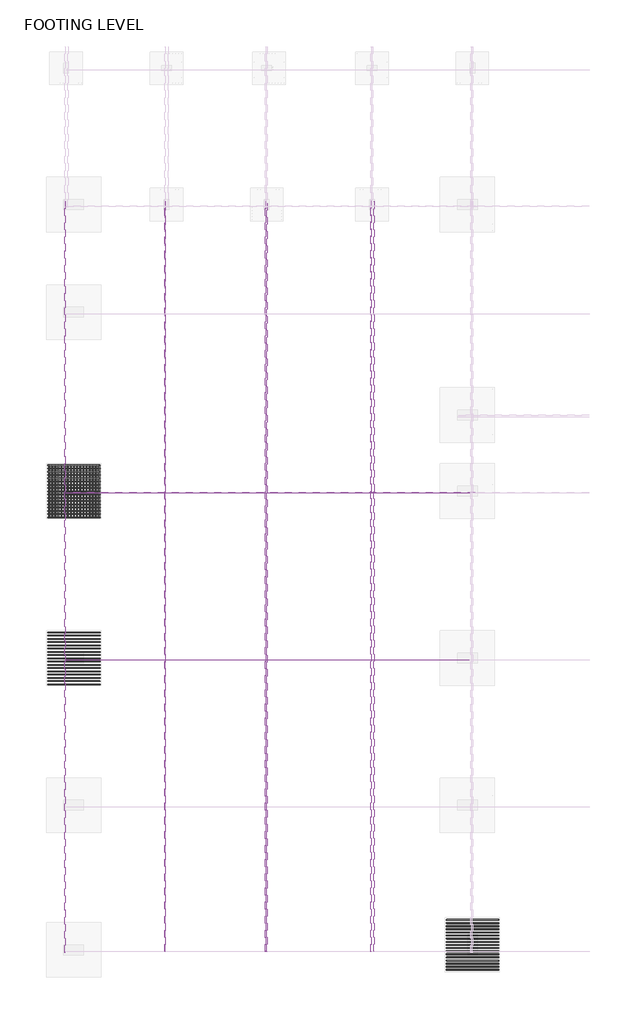
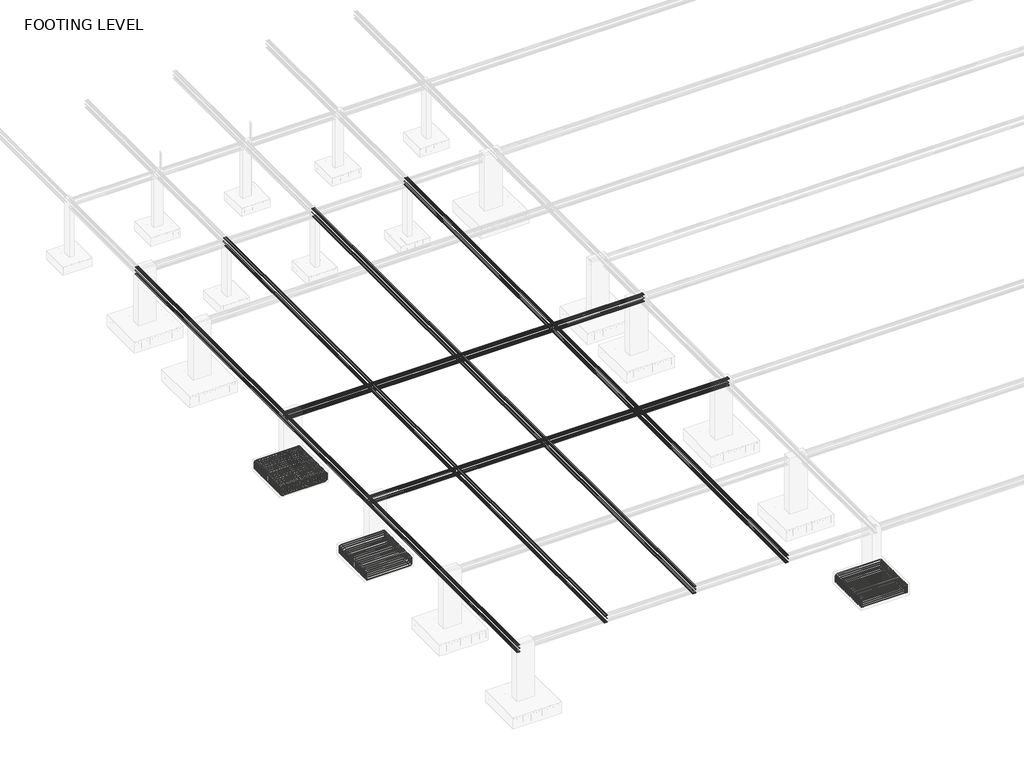
# One storey, part 4 of 19: 26 reinforcing bars.
"""IFC4 building model written with IfcOpenShell, lengths in millimetres."""

from ifc_helpers import new_model, si_unit, point, frame, origin, place, context, project, spatial, polyline, circle_curve, trimmed, segment, composite_curve, source, transform, mapped, element, save
from ifc_brep_helpers import swept_disk

model = new_model("IFC4")

# Units and contexts
model_context = context("Model", 3, world=origin())
ifc_project = project(units=[si_unit("LENGTHUNIT", "METRE", prefix="MILLI")], contexts=[model_context])

# Site, building, storey
site = spatial("IfcSite", under=ifc_project)
building = spatial("IfcBuilding", under=site)
storey = spatial("IfcBuildingStorey", under=building, Name="FOOTING LEVEL", Elevation=-3048.0)

# Reinforcing bars
placement = place(None, origin())
reinforcing_bar_shape = source(origin(), model_context, "Body", "SolidModel", [
    swept_disk(composite_curve([segment(polyline([(2562.6587563, -28952.7516566, -3148.0), (2562.6587563, -28952.7516566, -3470.1)]), True, "CONTINUOUS"), segment(trimmed(circle_curve(frame((2472.4587563, -28952.7516566, -3470.1), z_axis=(0.0, 1.0, 0.0), x_axis=(90.19999999999982, 0.0, 0.0)), 90.2), [point((2562.6587563, -28952.7516566, -3470.1))], [point((2472.4587563, -28952.7516566, -3560.3))], True, "CARTESIAN"), True, "CONTINUOUS"), segment(polyline([(2472.4587563, -28952.7516566, -3560.3), (278.2587563, -28952.7516566, -3560.3)]), True, "CONTINUOUS"), segment(trimmed(circle_curve(frame((278.2587563, -28952.7516566, -3470.1), z_axis=(0.0, 1.0, 0.0), x_axis=(0.0, 0.0, -90.20000000000027)), 90.2), [point((278.2587563, -28952.7516566, -3560.3))], [point((188.0587563, -28952.7516566, -3470.1))], True, "CARTESIAN"), True, "CONTINUOUS"), segment(polyline([(188.0587563, -28952.7516566, -3470.1), (188.0587563, -28952.7516566, -3148.0)]), True, "CONTINUOUS")], self_intersect=False), 12.7),
])
element("IfcReinforcingBar", 1, at=placement, inside=storey, context=model_context, shape_type="MappedRepresentation", body=[
    mapped(reinforcing_bar_shape, transform((0.0, 0.0, 0.0), x_axis=(1.0, 0.0, 0.0), y_axis=(0.0, 1.0, 0.0), z_axis=(0.0, 0.0, 1.0))),
    mapped(reinforcing_bar_shape, transform((0.0, 140.8090411, 0.0), x_axis=(1.0, 0.0, 0.0), y_axis=(0.0, 1.0, 0.0), z_axis=(0.0, 0.0, 1.0))),
    mapped(reinforcing_bar_shape, transform((0.0, 281.6180821, 0.0), x_axis=(1.0, 0.0, 0.0), y_axis=(0.0, 1.0, 0.0), z_axis=(0.0, 0.0, 1.0))),
    mapped(reinforcing_bar_shape, transform((0.0, 422.4271232, 0.0), x_axis=(1.0, 0.0, 0.0), y_axis=(0.0, 1.0, 0.0), z_axis=(0.0, 0.0, 1.0))),
    mapped(reinforcing_bar_shape, transform((0.0, 563.2361643, 0.0), x_axis=(1.0, 0.0, 0.0), y_axis=(0.0, 1.0, 0.0), z_axis=(0.0, 0.0, 1.0))),
    mapped(reinforcing_bar_shape, transform((0.0, 704.0452054, 0.0), x_axis=(1.0, 0.0, 0.0), y_axis=(0.0, 1.0, 0.0), z_axis=(0.0, 0.0, 1.0))),
    mapped(reinforcing_bar_shape, transform((0.0, 844.8542464, 0.0), x_axis=(1.0, 0.0, 0.0), y_axis=(0.0, 1.0, 0.0), z_axis=(0.0, 0.0, 1.0))),
    mapped(reinforcing_bar_shape, transform((0.0, 985.6632875, 0.0), x_axis=(1.0, 0.0, 0.0), y_axis=(0.0, 1.0, 0.0), z_axis=(0.0, 0.0, 1.0))),
    mapped(reinforcing_bar_shape, transform((0.0, 1126.4723286, 0.0), x_axis=(1.0, 0.0, 0.0), y_axis=(0.0, 1.0, 0.0), z_axis=(0.0, 0.0, 1.0))),
    mapped(reinforcing_bar_shape, transform((0.0, 1267.2813697, 0.0), x_axis=(1.0, 0.0, 0.0), y_axis=(0.0, 1.0, 0.0), z_axis=(0.0, 0.0, 1.0))),
    mapped(reinforcing_bar_shape, transform((0.0, 1408.0904107, 0.0), x_axis=(1.0, 0.0, 0.0), y_axis=(0.0, 1.0, 0.0), z_axis=(0.0, 0.0, 1.0))),
    mapped(reinforcing_bar_shape, transform((0.0, 1548.8994518, 0.0), x_axis=(1.0, 0.0, 0.0), y_axis=(0.0, 1.0, 0.0), z_axis=(0.0, 0.0, 1.0))),
    mapped(reinforcing_bar_shape, transform((0.0, 1689.7084929, 0.0), x_axis=(1.0, 0.0, 0.0), y_axis=(0.0, 1.0, 0.0), z_axis=(0.0, 0.0, 1.0))),
    mapped(reinforcing_bar_shape, transform((0.0, 1830.517534, 0.0), x_axis=(1.0, 0.0, 0.0), y_axis=(0.0, 1.0, 0.0), z_axis=(0.0, 0.0, 1.0))),
    mapped(reinforcing_bar_shape, transform((0.0, 1971.326575, 0.0), x_axis=(1.0, 0.0, 0.0), y_axis=(0.0, 1.0, 0.0), z_axis=(0.0, 0.0, 1.0))),
    mapped(reinforcing_bar_shape, transform((0.0, 2112.1356161, 0.0), x_axis=(1.0, 0.0, 0.0), y_axis=(0.0, 1.0, 0.0), z_axis=(0.0, 0.0, 1.0))),
    mapped(reinforcing_bar_shape, transform((0.0, 2252.9446572, 0.0), x_axis=(1.0, 0.0, 0.0), y_axis=(0.0, 1.0, 0.0), z_axis=(0.0, 0.0, 1.0))),
])
reinforcing_bar_2_shape = source(origin(), model_context, "Body", "SolidModel", [
    swept_disk(composite_curve([segment(polyline([(2562.6587563, -26677.3596072, -3548.0), (2562.6587563, -26677.3596072, -3225.9)]), True, "CONTINUOUS"), segment(trimmed(circle_curve(frame((2472.4587563, -26677.3596072, -3225.9), z_axis=(0.0, -1.0, 0.0), x_axis=(90.19999999999982, 0.0, 0.0)), 90.2), [point((2562.6587563, -26677.3596072, -3225.9))], [point((2472.4587563, -26677.3596072, -3135.7))], True, "CARTESIAN"), True, "CONTINUOUS"), segment(polyline([(2472.4587563, -26677.3596072, -3135.7), (278.2587563, -26677.3596072, -3135.7)]), True, "CONTINUOUS"), segment(trimmed(circle_curve(frame((278.2587563, -26677.3596072, -3225.9), z_axis=(0.0, -1.0, 0.0), x_axis=(0.0, 0.0, 90.20000000000027)), 90.2), [point((278.2587563, -26677.3596072, -3135.7))], [point((188.0587563, -26677.3596072, -3225.9))], True, "CARTESIAN"), True, "CONTINUOUS"), segment(polyline([(188.0587563, -26677.3596072, -3225.9), (188.0587563, -26677.3596072, -3548.0)]), True, "CONTINUOUS")], self_intersect=False), 12.7),
])
element("IfcReinforcingBar", 2, at=placement, inside=storey, context=model_context, shape_type="MappedRepresentation", body=[
    mapped(reinforcing_bar_2_shape, transform((0.0, 0.0, 0.0), x_axis=(1.0, 0.0, 0.0), y_axis=(0.0, 1.0, 0.0), z_axis=(0.0, 0.0, 1.0))),
    mapped(reinforcing_bar_2_shape, transform((0.0, -143.8496077, 0.0), x_axis=(1.0, 0.0, 0.0), y_axis=(0.0, 1.0, 0.0), z_axis=(0.0, 0.0, 1.0))),
    mapped(reinforcing_bar_2_shape, transform((0.0, -287.6992155, 0.0), x_axis=(1.0, 0.0, 0.0), y_axis=(0.0, 1.0, 0.0), z_axis=(0.0, 0.0, 1.0))),
    mapped(reinforcing_bar_2_shape, transform((0.0, -431.5488232, 0.0), x_axis=(1.0, 0.0, 0.0), y_axis=(0.0, 1.0, 0.0), z_axis=(0.0, 0.0, 1.0))),
    mapped(reinforcing_bar_2_shape, transform((0.0, -575.398431, 0.0), x_axis=(1.0, 0.0, 0.0), y_axis=(0.0, 1.0, 0.0), z_axis=(0.0, 0.0, 1.0))),
    mapped(reinforcing_bar_2_shape, transform((0.0, -719.2480387, 0.0), x_axis=(1.0, 0.0, 0.0), y_axis=(0.0, 1.0, 0.0), z_axis=(0.0, 0.0, 1.0))),
    mapped(reinforcing_bar_2_shape, transform((0.0, -863.0976465, 0.0), x_axis=(1.0, 0.0, 0.0), y_axis=(0.0, 1.0, 0.0), z_axis=(0.0, 0.0, 1.0))),
    mapped(reinforcing_bar_2_shape, transform((0.0, -1006.9472542, 0.0), x_axis=(1.0, 0.0, 0.0), y_axis=(0.0, 1.0, 0.0), z_axis=(0.0, 0.0, 1.0))),
    mapped(reinforcing_bar_2_shape, transform((0.0, -1150.796862, 0.0), x_axis=(1.0, 0.0, 0.0), y_axis=(0.0, 1.0, 0.0), z_axis=(0.0, 0.0, 1.0))),
    mapped(reinforcing_bar_2_shape, transform((0.0, -1294.6464697, 0.0), x_axis=(1.0, 0.0, 0.0), y_axis=(0.0, 1.0, 0.0), z_axis=(0.0, 0.0, 1.0))),
    mapped(reinforcing_bar_2_shape, transform((0.0, -1438.4960775, 0.0), x_axis=(1.0, 0.0, 0.0), y_axis=(0.0, 1.0, 0.0), z_axis=(0.0, 0.0, 1.0))),
    mapped(reinforcing_bar_2_shape, transform((0.0, -1582.3456852, 0.0), x_axis=(1.0, 0.0, 0.0), y_axis=(0.0, 1.0, 0.0), z_axis=(0.0, 0.0, 1.0))),
    mapped(reinforcing_bar_2_shape, transform((0.0, -1726.195293, 0.0), x_axis=(1.0, 0.0, 0.0), y_axis=(0.0, 1.0, 0.0), z_axis=(0.0, 0.0, 1.0))),
    mapped(reinforcing_bar_2_shape, transform((0.0, -1870.0449007, 0.0), x_axis=(1.0, 0.0, 0.0), y_axis=(0.0, 1.0, 0.0), z_axis=(0.0, 0.0, 1.0))),
    mapped(reinforcing_bar_2_shape, transform((0.0, -2013.8945085, 0.0), x_axis=(1.0, 0.0, 0.0), y_axis=(0.0, 1.0, 0.0), z_axis=(0.0, 0.0, 1.0))),
    mapped(reinforcing_bar_2_shape, transform((0.0, -2157.7441162, 0.0), x_axis=(1.0, 0.0, 0.0), y_axis=(0.0, 1.0, 0.0), z_axis=(0.0, 0.0, 1.0))),
    mapped(reinforcing_bar_2_shape, transform((0.0, -2301.5937239, 0.0), x_axis=(1.0, 0.0, 0.0), y_axis=(0.0, 1.0, 0.0), z_axis=(0.0, 0.0, 1.0))),
])
reinforcing_bar_3_shape = source(origin(), model_context, "Body", "SolidModel", [
    swept_disk(composite_curve([segment(polyline([(-17985.6412437, -13575.4205555, -3173.0), (-17985.6412437, -13575.4205555, -3495.1)]), True, "CONTINUOUS"), segment(trimmed(circle_curve(frame((-17895.4412437, -13575.4205555, -3495.1), z_axis=(0.0, -1.0, 0.0), x_axis=(-90.20000000000073, 0.0, 0.0)), 90.2), [point((-17985.6412437, -13575.4205555, -3495.1))], [point((-17895.4412437, -13575.4205555, -3585.3))], True, "CARTESIAN"), True, "CONTINUOUS"), segment(polyline([(-17895.4412437, -13575.4205555, -3585.3), (-15701.2412437, -13575.4205555, -3585.3)]), True, "CONTINUOUS"), segment(trimmed(circle_curve(frame((-15701.2412437, -13575.4205555, -3495.1), z_axis=(0.0, -1.0, 0.0), x_axis=(0.0, 0.0, -90.20000000000027)), 90.2), [point((-15701.2412437, -13575.4205555, -3585.3))], [point((-15611.0412437, -13575.4205555, -3495.1))], True, "CARTESIAN"), True, "CONTINUOUS"), segment(polyline([(-15611.0412437, -13575.4205555, -3495.1), (-15611.0412437, -13575.4205555, -3173.0)]), True, "CONTINUOUS")], self_intersect=False), 12.7),
])
element("IfcReinforcingBar", 3, at=placement, inside=storey, context=model_context, shape_type="MappedRepresentation", body=[
    mapped(reinforcing_bar_3_shape, transform((0.0, 0.0, 0.0), x_axis=(1.0, 0.0, 0.0), y_axis=(0.0, 1.0, 0.0), z_axis=(0.0, 0.0, 1.0))),
    mapped(reinforcing_bar_3_shape, transform((0.0, -148.4125, 0.0), x_axis=(1.0, 0.0, 0.0), y_axis=(0.0, 1.0, 0.0), z_axis=(0.0, 0.0, 1.0))),
    mapped(reinforcing_bar_3_shape, transform((0.0, -296.825, 0.0), x_axis=(1.0, 0.0, 0.0), y_axis=(0.0, 1.0, 0.0), z_axis=(0.0, 0.0, 1.0))),
    mapped(reinforcing_bar_3_shape, transform((0.0, -445.2375, 0.0), x_axis=(1.0, 0.0, 0.0), y_axis=(0.0, 1.0, 0.0), z_axis=(0.0, 0.0, 1.0))),
    mapped(reinforcing_bar_3_shape, transform((0.0, -593.65, 0.0), x_axis=(1.0, 0.0, 0.0), y_axis=(0.0, 1.0, 0.0), z_axis=(0.0, 0.0, 1.0))),
    mapped(reinforcing_bar_3_shape, transform((0.0, -742.0625, 0.0), x_axis=(1.0, 0.0, 0.0), y_axis=(0.0, 1.0, 0.0), z_axis=(0.0, 0.0, 1.0))),
    mapped(reinforcing_bar_3_shape, transform((0.0, -890.475, 0.0), x_axis=(1.0, 0.0, 0.0), y_axis=(0.0, 1.0, 0.0), z_axis=(0.0, 0.0, 1.0))),
    mapped(reinforcing_bar_3_shape, transform((0.0, -1038.8875, 0.0), x_axis=(1.0, 0.0, 0.0), y_axis=(0.0, 1.0, 0.0), z_axis=(0.0, 0.0, 1.0))),
    mapped(reinforcing_bar_3_shape, transform((0.0, -1187.3, 0.0), x_axis=(1.0, 0.0, 0.0), y_axis=(0.0, 1.0, 0.0), z_axis=(0.0, 0.0, 1.0))),
    mapped(reinforcing_bar_3_shape, transform((0.0, -1335.7125, 0.0), x_axis=(1.0, 0.0, 0.0), y_axis=(0.0, 1.0, 0.0), z_axis=(0.0, 0.0, 1.0))),
    mapped(reinforcing_bar_3_shape, transform((0.0, -1484.125, 0.0), x_axis=(1.0, 0.0, 0.0), y_axis=(0.0, 1.0, 0.0), z_axis=(0.0, 0.0, 1.0))),
    mapped(reinforcing_bar_3_shape, transform((0.0, -1632.5375, 0.0), x_axis=(1.0, 0.0, 0.0), y_axis=(0.0, 1.0, 0.0), z_axis=(0.0, 0.0, 1.0))),
    mapped(reinforcing_bar_3_shape, transform((0.0, -1780.95, 0.0), x_axis=(1.0, 0.0, 0.0), y_axis=(0.0, 1.0, 0.0), z_axis=(0.0, 0.0, 1.0))),
    mapped(reinforcing_bar_3_shape, transform((0.0, -1929.3625, 0.0), x_axis=(1.0, 0.0, 0.0), y_axis=(0.0, 1.0, 0.0), z_axis=(0.0, 0.0, 1.0))),
    mapped(reinforcing_bar_3_shape, transform((0.0, -2077.775, 0.0), x_axis=(1.0, 0.0, 0.0), y_axis=(0.0, 1.0, 0.0), z_axis=(0.0, 0.0, 1.0))),
    mapped(reinforcing_bar_3_shape, transform((0.0, -2226.1875, 0.0), x_axis=(1.0, 0.0, 0.0), y_axis=(0.0, 1.0, 0.0), z_axis=(0.0, 0.0, 1.0))),
    mapped(reinforcing_bar_3_shape, transform((0.0, -2374.6, 0.0), x_axis=(1.0, 0.0, 0.0), y_axis=(0.0, 1.0, 0.0), z_axis=(0.0, 0.0, 1.0))),
])
reinforcing_bar_4_shape = source(origin(), model_context, "Body", "SolidModel", [
    swept_disk(composite_curve([segment(polyline([(-15611.0412437, -13575.4205555, -3523.0), (-15611.0412437, -13575.4205555, -3200.9)]), True, "CONTINUOUS"), segment(trimmed(circle_curve(frame((-15701.2412437, -13575.4205555, -3200.9), z_axis=(0.0, -1.0, 0.0), x_axis=(90.20000000000073, 0.0, 0.0)), 90.2), [point((-15611.0412437, -13575.4205555, -3200.9))], [point((-15701.2412437, -13575.4205555, -3110.7))], True, "CARTESIAN"), True, "CONTINUOUS"), segment(polyline([(-15701.2412437, -13575.4205555, -3110.7), (-17895.4412437, -13575.4205555, -3110.7)]), True, "CONTINUOUS"), segment(trimmed(circle_curve(frame((-17895.4412437, -13575.4205555, -3200.9), z_axis=(0.0, -1.0, 0.0), x_axis=(0.0, 0.0, 90.20000000000027)), 90.2), [point((-17895.4412437, -13575.4205555, -3110.7))], [point((-17985.6412437, -13575.4205555, -3200.9))], True, "CARTESIAN"), True, "CONTINUOUS"), segment(polyline([(-17985.6412437, -13575.4205555, -3200.9), (-17985.6412437, -13575.4205555, -3523.0)]), True, "CONTINUOUS")], self_intersect=False), 12.7),
])
element("IfcReinforcingBar", 4, at=placement, inside=storey, context=model_context, shape_type="MappedRepresentation", body=[
    mapped(reinforcing_bar_4_shape, transform((0.0, 0.0, 0.0), x_axis=(1.0, 0.0, 0.0), y_axis=(0.0, 1.0, 0.0), z_axis=(0.0, 0.0, 1.0))),
    mapped(reinforcing_bar_4_shape, transform((0.0, -148.4125, 0.0), x_axis=(1.0, 0.0, 0.0), y_axis=(0.0, 1.0, 0.0), z_axis=(0.0, 0.0, 1.0))),
    mapped(reinforcing_bar_4_shape, transform((0.0, -296.825, 0.0), x_axis=(1.0, 0.0, 0.0), y_axis=(0.0, 1.0, 0.0), z_axis=(0.0, 0.0, 1.0))),
    mapped(reinforcing_bar_4_shape, transform((0.0, -445.2375, 0.0), x_axis=(1.0, 0.0, 0.0), y_axis=(0.0, 1.0, 0.0), z_axis=(0.0, 0.0, 1.0))),
    mapped(reinforcing_bar_4_shape, transform((0.0, -593.65, 0.0), x_axis=(1.0, 0.0, 0.0), y_axis=(0.0, 1.0, 0.0), z_axis=(0.0, 0.0, 1.0))),
    mapped(reinforcing_bar_4_shape, transform((0.0, -742.0625, 0.0), x_axis=(1.0, 0.0, 0.0), y_axis=(0.0, 1.0, 0.0), z_axis=(0.0, 0.0, 1.0))),
    mapped(reinforcing_bar_4_shape, transform((0.0, -890.475, 0.0), x_axis=(1.0, 0.0, 0.0), y_axis=(0.0, 1.0, 0.0), z_axis=(0.0, 0.0, 1.0))),
    mapped(reinforcing_bar_4_shape, transform((0.0, -1038.8875, 0.0), x_axis=(1.0, 0.0, 0.0), y_axis=(0.0, 1.0, 0.0), z_axis=(0.0, 0.0, 1.0))),
    mapped(reinforcing_bar_4_shape, transform((0.0, -1187.3, 0.0), x_axis=(1.0, 0.0, 0.0), y_axis=(0.0, 1.0, 0.0), z_axis=(0.0, 0.0, 1.0))),
    mapped(reinforcing_bar_4_shape, transform((0.0, -1335.7125, 0.0), x_axis=(1.0, 0.0, 0.0), y_axis=(0.0, 1.0, 0.0), z_axis=(0.0, 0.0, 1.0))),
    mapped(reinforcing_bar_4_shape, transform((0.0, -1484.125, 0.0), x_axis=(1.0, 0.0, 0.0), y_axis=(0.0, 1.0, 0.0), z_axis=(0.0, 0.0, 1.0))),
    mapped(reinforcing_bar_4_shape, transform((0.0, -1632.5375, 0.0), x_axis=(1.0, 0.0, 0.0), y_axis=(0.0, 1.0, 0.0), z_axis=(0.0, 0.0, 1.0))),
    mapped(reinforcing_bar_4_shape, transform((0.0, -1780.95, 0.0), x_axis=(1.0, 0.0, 0.0), y_axis=(0.0, 1.0, 0.0), z_axis=(0.0, 0.0, 1.0))),
    mapped(reinforcing_bar_4_shape, transform((0.0, -1929.3625, 0.0), x_axis=(1.0, 0.0, 0.0), y_axis=(0.0, 1.0, 0.0), z_axis=(0.0, 0.0, 1.0))),
    mapped(reinforcing_bar_4_shape, transform((0.0, -2077.775, 0.0), x_axis=(1.0, 0.0, 0.0), y_axis=(0.0, 1.0, 0.0), z_axis=(0.0, 0.0, 1.0))),
    mapped(reinforcing_bar_4_shape, transform((0.0, -2226.1875, 0.0), x_axis=(1.0, 0.0, 0.0), y_axis=(0.0, 1.0, 0.0), z_axis=(0.0, 0.0, 1.0))),
    mapped(reinforcing_bar_4_shape, transform((0.0, -2374.6, 0.0), x_axis=(1.0, 0.0, 0.0), y_axis=(0.0, 1.0, 0.0), z_axis=(0.0, 0.0, 1.0))),
])
reinforcing_bar_5_shape = source(origin(), model_context, "Body", "SolidModel", [
    swept_disk(composite_curve([segment(polyline([(-17920.0723448, -8330.0205555, -3148.0), (-17920.0723448, -8330.0205555, -3470.1)]), True, "CONTINUOUS"), segment(trimmed(circle_curve(frame((-17920.0723448, -8239.8205555, -3470.1), z_axis=(1.0, 0.0, 0.0), x_axis=(0.0, -90.19999999999891, 0.0)), 90.2), [point((-17920.0723448, -8330.0205555, -3470.1))], [point((-17920.0723448, -8239.8205555, -3560.3))], True, "CARTESIAN"), True, "CONTINUOUS"), segment(polyline([(-17920.0723448, -8239.8205555, -3560.3), (-17920.0723448, -6045.6205555, -3560.3)]), True, "CONTINUOUS"), segment(trimmed(circle_curve(frame((-17920.0723448, -6045.6205555, -3470.1), z_axis=(1.0, 0.0, 0.0), x_axis=(0.0, 0.0, -90.20000000000027)), 90.2), [point((-17920.0723448, -6045.6205555, -3560.3))], [point((-17920.0723448, -5955.4205555, -3470.1))], True, "CARTESIAN"), True, "CONTINUOUS"), segment(polyline([(-17920.0723448, -5955.4205555, -3470.1), (-17920.0723448, -5955.4205555, -3148.0)]), True, "CONTINUOUS")], self_intersect=False), 12.7),
])
element("IfcReinforcingBar", 5, at=placement, inside=storey, context=model_context, shape_type="MappedRepresentation", body=[
    mapped(reinforcing_bar_5_shape, transform((0.0, 0.0, 0.0), x_axis=(1.0, 0.0, 0.0), y_axis=(0.0, 1.0, 0.0), z_axis=(0.0, 0.0, 1.0))),
    mapped(reinforcing_bar_5_shape, transform((140.8090411, 0.0, 0.0), x_axis=(1.0, 0.0, 0.0), y_axis=(0.0, 1.0, 0.0), z_axis=(0.0, 0.0, 1.0))),
    mapped(reinforcing_bar_5_shape, transform((281.6180821, 0.0, 0.0), x_axis=(1.0, 0.0, 0.0), y_axis=(0.0, 1.0, 0.0), z_axis=(0.0, 0.0, 1.0))),
    mapped(reinforcing_bar_5_shape, transform((422.4271232, 0.0, 0.0), x_axis=(1.0, 0.0, 0.0), y_axis=(0.0, 1.0, 0.0), z_axis=(0.0, 0.0, 1.0))),
    mapped(reinforcing_bar_5_shape, transform((563.2361643, 0.0, 0.0), x_axis=(1.0, 0.0, 0.0), y_axis=(0.0, 1.0, 0.0), z_axis=(0.0, 0.0, 1.0))),
    mapped(reinforcing_bar_5_shape, transform((704.0452054, 0.0, 0.0), x_axis=(1.0, 0.0, 0.0), y_axis=(0.0, 1.0, 0.0), z_axis=(0.0, 0.0, 1.0))),
    mapped(reinforcing_bar_5_shape, transform((844.8542464, 0.0, 0.0), x_axis=(1.0, 0.0, 0.0), y_axis=(0.0, 1.0, 0.0), z_axis=(0.0, 0.0, 1.0))),
    mapped(reinforcing_bar_5_shape, transform((985.6632875, 0.0, 0.0), x_axis=(1.0, 0.0, 0.0), y_axis=(0.0, 1.0, 0.0), z_axis=(0.0, 0.0, 1.0))),
    mapped(reinforcing_bar_5_shape, transform((1126.4723286, 0.0, 0.0), x_axis=(1.0, 0.0, 0.0), y_axis=(0.0, 1.0, 0.0), z_axis=(0.0, 0.0, 1.0))),
    mapped(reinforcing_bar_5_shape, transform((1267.2813697, 0.0, 0.0), x_axis=(1.0, 0.0, 0.0), y_axis=(0.0, 1.0, 0.0), z_axis=(0.0, 0.0, 1.0))),
    mapped(reinforcing_bar_5_shape, transform((1408.0904107, 0.0, 0.0), x_axis=(1.0, 0.0, 0.0), y_axis=(0.0, 1.0, 0.0), z_axis=(0.0, 0.0, 1.0))),
    mapped(reinforcing_bar_5_shape, transform((1548.8994518, 0.0, 0.0), x_axis=(1.0, 0.0, 0.0), y_axis=(0.0, 1.0, 0.0), z_axis=(0.0, 0.0, 1.0))),
    mapped(reinforcing_bar_5_shape, transform((1689.7084929, 0.0, 0.0), x_axis=(1.0, 0.0, 0.0), y_axis=(0.0, 1.0, 0.0), z_axis=(0.0, 0.0, 1.0))),
    mapped(reinforcing_bar_5_shape, transform((1830.517534, 0.0, 0.0), x_axis=(1.0, 0.0, 0.0), y_axis=(0.0, 1.0, 0.0), z_axis=(0.0, 0.0, 1.0))),
    mapped(reinforcing_bar_5_shape, transform((1971.326575, 0.0, 0.0), x_axis=(1.0, 0.0, 0.0), y_axis=(0.0, 1.0, 0.0), z_axis=(0.0, 0.0, 1.0))),
    mapped(reinforcing_bar_5_shape, transform((2112.1356161, 0.0, 0.0), x_axis=(1.0, 0.0, 0.0), y_axis=(0.0, 1.0, 0.0), z_axis=(0.0, 0.0, 1.0))),
    mapped(reinforcing_bar_5_shape, transform((2252.9446572, 0.0, 0.0), x_axis=(1.0, 0.0, 0.0), y_axis=(0.0, 1.0, 0.0), z_axis=(0.0, 0.0, 1.0))),
])
reinforcing_bar_6_shape = source(origin(), model_context, "Body", "SolidModel", [
    swept_disk(composite_curve([segment(polyline([(-15644.6802955, -8330.0205555, -3548.0), (-15644.6802955, -8330.0205555, -3225.9)]), True, "CONTINUOUS"), segment(trimmed(circle_curve(frame((-15644.6802955, -8239.8205555, -3225.9), z_axis=(-1.0, 0.0, 0.0), x_axis=(0.0, -90.19999999999891, 0.0)), 90.2), [point((-15644.6802955, -8330.0205555, -3225.9))], [point((-15644.6802955, -8239.8205555, -3135.7))], True, "CARTESIAN"), True, "CONTINUOUS"), segment(polyline([(-15644.6802955, -8239.8205555, -3135.7), (-15644.6802955, -6045.6205555, -3135.7)]), True, "CONTINUOUS"), segment(trimmed(circle_curve(frame((-15644.6802955, -6045.6205555, -3225.9), z_axis=(-1.0, 0.0, 0.0), x_axis=(0.0, 0.0, 90.20000000000027)), 90.2), [point((-15644.6802955, -6045.6205555, -3135.7))], [point((-15644.6802955, -5955.4205555, -3225.9))], True, "CARTESIAN"), True, "CONTINUOUS"), segment(polyline([(-15644.6802955, -5955.4205555, -3225.9), (-15644.6802955, -5955.4205555, -3548.0)]), True, "CONTINUOUS")], self_intersect=False), 12.7),
])
element("IfcReinforcingBar", 6, at=placement, inside=storey, context=model_context, shape_type="MappedRepresentation", body=[
    mapped(reinforcing_bar_6_shape, transform((0.0, 0.0, 0.0), x_axis=(1.0, 0.0, 0.0), y_axis=(0.0, 1.0, 0.0), z_axis=(0.0, 0.0, 1.0))),
    mapped(reinforcing_bar_6_shape, transform((-143.8496077, 0.0, 0.0), x_axis=(1.0, 0.0, 0.0), y_axis=(0.0, 1.0, 0.0), z_axis=(0.0, 0.0, 1.0))),
    mapped(reinforcing_bar_6_shape, transform((-287.6992155, 0.0, 0.0), x_axis=(1.0, 0.0, 0.0), y_axis=(0.0, 1.0, 0.0), z_axis=(0.0, 0.0, 1.0))),
    mapped(reinforcing_bar_6_shape, transform((-431.5488232, 0.0, 0.0), x_axis=(1.0, 0.0, 0.0), y_axis=(0.0, 1.0, 0.0), z_axis=(0.0, 0.0, 1.0))),
    mapped(reinforcing_bar_6_shape, transform((-575.398431, 0.0, 0.0), x_axis=(1.0, 0.0, 0.0), y_axis=(0.0, 1.0, 0.0), z_axis=(0.0, 0.0, 1.0))),
    mapped(reinforcing_bar_6_shape, transform((-719.2480387, 0.0, 0.0), x_axis=(1.0, 0.0, 0.0), y_axis=(0.0, 1.0, 0.0), z_axis=(0.0, 0.0, 1.0))),
    mapped(reinforcing_bar_6_shape, transform((-863.0976465, 0.0, 0.0), x_axis=(1.0, 0.0, 0.0), y_axis=(0.0, 1.0, 0.0), z_axis=(0.0, 0.0, 1.0))),
    mapped(reinforcing_bar_6_shape, transform((-1006.9472542, 0.0, 0.0), x_axis=(1.0, 0.0, 0.0), y_axis=(0.0, 1.0, 0.0), z_axis=(0.0, 0.0, 1.0))),
    mapped(reinforcing_bar_6_shape, transform((-1150.796862, 0.0, 0.0), x_axis=(1.0, 0.0, 0.0), y_axis=(0.0, 1.0, 0.0), z_axis=(0.0, 0.0, 1.0))),
    mapped(reinforcing_bar_6_shape, transform((-1294.6464697, 0.0, 0.0), x_axis=(1.0, 0.0, 0.0), y_axis=(0.0, 1.0, 0.0), z_axis=(0.0, 0.0, 1.0))),
    mapped(reinforcing_bar_6_shape, transform((-1438.4960775, 0.0, 0.0), x_axis=(1.0, 0.0, 0.0), y_axis=(0.0, 1.0, 0.0), z_axis=(0.0, 0.0, 1.0))),
    mapped(reinforcing_bar_6_shape, transform((-1582.3456852, 0.0, 0.0), x_axis=(1.0, 0.0, 0.0), y_axis=(0.0, 1.0, 0.0), z_axis=(0.0, 0.0, 1.0))),
    mapped(reinforcing_bar_6_shape, transform((-1726.195293, 0.0, 0.0), x_axis=(1.0, 0.0, 0.0), y_axis=(0.0, 1.0, 0.0), z_axis=(0.0, 0.0, 1.0))),
    mapped(reinforcing_bar_6_shape, transform((-1870.0449007, 0.0, 0.0), x_axis=(1.0, 0.0, 0.0), y_axis=(0.0, 1.0, 0.0), z_axis=(0.0, 0.0, 1.0))),
    mapped(reinforcing_bar_6_shape, transform((-2013.8945085, 0.0, 0.0), x_axis=(1.0, 0.0, 0.0), y_axis=(0.0, 1.0, 0.0), z_axis=(0.0, 0.0, 1.0))),
    mapped(reinforcing_bar_6_shape, transform((-2157.7441162, 0.0, 0.0), x_axis=(1.0, 0.0, 0.0), y_axis=(0.0, 1.0, 0.0), z_axis=(0.0, 0.0, 1.0))),
    mapped(reinforcing_bar_6_shape, transform((-2301.5937239, 0.0, 0.0), x_axis=(1.0, 0.0, 0.0), y_axis=(0.0, 1.0, 0.0), z_axis=(0.0, 0.0, 1.0))),
])
reinforcing_bar_7_shape = source(origin(), model_context, "Body", "SolidModel", [
    swept_disk(composite_curve([segment(polyline([(-17985.6412437, -5955.4205555, -3173.0), (-17985.6412437, -5955.4205555, -3495.1)]), True, "CONTINUOUS"), segment(trimmed(circle_curve(frame((-17895.4412437, -5955.4205555, -3495.1), z_axis=(0.0, -1.0, 0.0), x_axis=(-90.20000000000073, 0.0, 0.0)), 90.2), [point((-17985.6412437, -5955.4205555, -3495.1))], [point((-17895.4412437, -5955.4205555, -3585.3))], True, "CARTESIAN"), True, "CONTINUOUS"), segment(polyline([(-17895.4412437, -5955.4205555, -3585.3), (-15701.2412437, -5955.4205555, -3585.3)]), True, "CONTINUOUS"), segment(trimmed(circle_curve(frame((-15701.2412437, -5955.4205555, -3495.1), z_axis=(0.0, -1.0, 0.0), x_axis=(0.0, 0.0, -90.20000000000027)), 90.2), [point((-15701.2412437, -5955.4205555, -3585.3))], [point((-15611.0412437, -5955.4205555, -3495.1))], True, "CARTESIAN"), True, "CONTINUOUS"), segment(polyline([(-15611.0412437, -5955.4205555, -3495.1), (-15611.0412437, -5955.4205555, -3173.0)]), True, "CONTINUOUS")], self_intersect=False), 12.7),
])
element("IfcReinforcingBar", 7, at=placement, inside=storey, context=model_context, shape_type="MappedRepresentation", body=[
    mapped(reinforcing_bar_7_shape, transform((0.0, 0.0, 0.0), x_axis=(1.0, 0.0, 0.0), y_axis=(0.0, 1.0, 0.0), z_axis=(0.0, 0.0, 1.0))),
    mapped(reinforcing_bar_7_shape, transform((0.0, -148.4125, 0.0), x_axis=(1.0, 0.0, 0.0), y_axis=(0.0, 1.0, 0.0), z_axis=(0.0, 0.0, 1.0))),
    mapped(reinforcing_bar_7_shape, transform((0.0, -296.825, 0.0), x_axis=(1.0, 0.0, 0.0), y_axis=(0.0, 1.0, 0.0), z_axis=(0.0, 0.0, 1.0))),
    mapped(reinforcing_bar_7_shape, transform((0.0, -445.2375, 0.0), x_axis=(1.0, 0.0, 0.0), y_axis=(0.0, 1.0, 0.0), z_axis=(0.0, 0.0, 1.0))),
    mapped(reinforcing_bar_7_shape, transform((0.0, -593.65, 0.0), x_axis=(1.0, 0.0, 0.0), y_axis=(0.0, 1.0, 0.0), z_axis=(0.0, 0.0, 1.0))),
    mapped(reinforcing_bar_7_shape, transform((0.0, -742.0625, 0.0), x_axis=(1.0, 0.0, 0.0), y_axis=(0.0, 1.0, 0.0), z_axis=(0.0, 0.0, 1.0))),
    mapped(reinforcing_bar_7_shape, transform((0.0, -890.475, 0.0), x_axis=(1.0, 0.0, 0.0), y_axis=(0.0, 1.0, 0.0), z_axis=(0.0, 0.0, 1.0))),
    mapped(reinforcing_bar_7_shape, transform((0.0, -1038.8875, 0.0), x_axis=(1.0, 0.0, 0.0), y_axis=(0.0, 1.0, 0.0), z_axis=(0.0, 0.0, 1.0))),
    mapped(reinforcing_bar_7_shape, transform((0.0, -1187.3, 0.0), x_axis=(1.0, 0.0, 0.0), y_axis=(0.0, 1.0, 0.0), z_axis=(0.0, 0.0, 1.0))),
    mapped(reinforcing_bar_7_shape, transform((0.0, -1335.7125, 0.0), x_axis=(1.0, 0.0, 0.0), y_axis=(0.0, 1.0, 0.0), z_axis=(0.0, 0.0, 1.0))),
    mapped(reinforcing_bar_7_shape, transform((0.0, -1484.125, 0.0), x_axis=(1.0, 0.0, 0.0), y_axis=(0.0, 1.0, 0.0), z_axis=(0.0, 0.0, 1.0))),
    mapped(reinforcing_bar_7_shape, transform((0.0, -1632.5375, 0.0), x_axis=(1.0, 0.0, 0.0), y_axis=(0.0, 1.0, 0.0), z_axis=(0.0, 0.0, 1.0))),
    mapped(reinforcing_bar_7_shape, transform((0.0, -1780.95, 0.0), x_axis=(1.0, 0.0, 0.0), y_axis=(0.0, 1.0, 0.0), z_axis=(0.0, 0.0, 1.0))),
    mapped(reinforcing_bar_7_shape, transform((0.0, -1929.3625, 0.0), x_axis=(1.0, 0.0, 0.0), y_axis=(0.0, 1.0, 0.0), z_axis=(0.0, 0.0, 1.0))),
    mapped(reinforcing_bar_7_shape, transform((0.0, -2077.775, 0.0), x_axis=(1.0, 0.0, 0.0), y_axis=(0.0, 1.0, 0.0), z_axis=(0.0, 0.0, 1.0))),
    mapped(reinforcing_bar_7_shape, transform((0.0, -2226.1875, 0.0), x_axis=(1.0, 0.0, 0.0), y_axis=(0.0, 1.0, 0.0), z_axis=(0.0, 0.0, 1.0))),
    mapped(reinforcing_bar_7_shape, transform((0.0, -2374.6, 0.0), x_axis=(1.0, 0.0, 0.0), y_axis=(0.0, 1.0, 0.0), z_axis=(0.0, 0.0, 1.0))),
])
reinforcing_bar_8_shape = source(origin(), model_context, "Body", "SolidModel", [
    swept_disk(composite_curve([segment(polyline([(-15611.0412437, -5955.4205555, -3523.0), (-15611.0412437, -5955.4205555, -3200.9)]), True, "CONTINUOUS"), segment(trimmed(circle_curve(frame((-15701.2412437, -5955.4205555, -3200.9), z_axis=(0.0, -1.0, 0.0), x_axis=(90.20000000000073, 0.0, 0.0)), 90.2), [point((-15611.0412437, -5955.4205555, -3200.9))], [point((-15701.2412437, -5955.4205555, -3110.7))], True, "CARTESIAN"), True, "CONTINUOUS"), segment(polyline([(-15701.2412437, -5955.4205555, -3110.7), (-17895.4412437, -5955.4205555, -3110.7)]), True, "CONTINUOUS"), segment(trimmed(circle_curve(frame((-17895.4412437, -5955.4205555, -3200.9), z_axis=(0.0, -1.0, 0.0), x_axis=(0.0, 0.0, 90.20000000000027)), 90.2), [point((-17895.4412437, -5955.4205555, -3110.7))], [point((-17985.6412437, -5955.4205555, -3200.9))], True, "CARTESIAN"), True, "CONTINUOUS"), segment(polyline([(-17985.6412437, -5955.4205555, -3200.9), (-17985.6412437, -5955.4205555, -3523.0)]), True, "CONTINUOUS")], self_intersect=False), 12.7),
])
element("IfcReinforcingBar", 8, at=placement, inside=storey, context=model_context, shape_type="MappedRepresentation", body=[
    mapped(reinforcing_bar_8_shape, transform((0.0, 0.0, 0.0), x_axis=(1.0, 0.0, 0.0), y_axis=(0.0, 1.0, 0.0), z_axis=(0.0, 0.0, 1.0))),
    mapped(reinforcing_bar_8_shape, transform((0.0, -148.4125, 0.0), x_axis=(1.0, 0.0, 0.0), y_axis=(0.0, 1.0, 0.0), z_axis=(0.0, 0.0, 1.0))),
    mapped(reinforcing_bar_8_shape, transform((0.0, -296.825, 0.0), x_axis=(1.0, 0.0, 0.0), y_axis=(0.0, 1.0, 0.0), z_axis=(0.0, 0.0, 1.0))),
    mapped(reinforcing_bar_8_shape, transform((0.0, -445.2375, 0.0), x_axis=(1.0, 0.0, 0.0), y_axis=(0.0, 1.0, 0.0), z_axis=(0.0, 0.0, 1.0))),
    mapped(reinforcing_bar_8_shape, transform((0.0, -593.65, 0.0), x_axis=(1.0, 0.0, 0.0), y_axis=(0.0, 1.0, 0.0), z_axis=(0.0, 0.0, 1.0))),
    mapped(reinforcing_bar_8_shape, transform((0.0, -742.0625, 0.0), x_axis=(1.0, 0.0, 0.0), y_axis=(0.0, 1.0, 0.0), z_axis=(0.0, 0.0, 1.0))),
    mapped(reinforcing_bar_8_shape, transform((0.0, -890.475, 0.0), x_axis=(1.0, 0.0, 0.0), y_axis=(0.0, 1.0, 0.0), z_axis=(0.0, 0.0, 1.0))),
    mapped(reinforcing_bar_8_shape, transform((0.0, -1038.8875, 0.0), x_axis=(1.0, 0.0, 0.0), y_axis=(0.0, 1.0, 0.0), z_axis=(0.0, 0.0, 1.0))),
    mapped(reinforcing_bar_8_shape, transform((0.0, -1187.3, 0.0), x_axis=(1.0, 0.0, 0.0), y_axis=(0.0, 1.0, 0.0), z_axis=(0.0, 0.0, 1.0))),
    mapped(reinforcing_bar_8_shape, transform((0.0, -1335.7125, 0.0), x_axis=(1.0, 0.0, 0.0), y_axis=(0.0, 1.0, 0.0), z_axis=(0.0, 0.0, 1.0))),
    mapped(reinforcing_bar_8_shape, transform((0.0, -1484.125, 0.0), x_axis=(1.0, 0.0, 0.0), y_axis=(0.0, 1.0, 0.0), z_axis=(0.0, 0.0, 1.0))),
    mapped(reinforcing_bar_8_shape, transform((0.0, -1632.5375, 0.0), x_axis=(1.0, 0.0, 0.0), y_axis=(0.0, 1.0, 0.0), z_axis=(0.0, 0.0, 1.0))),
    mapped(reinforcing_bar_8_shape, transform((0.0, -1780.95, 0.0), x_axis=(1.0, 0.0, 0.0), y_axis=(0.0, 1.0, 0.0), z_axis=(0.0, 0.0, 1.0))),
    mapped(reinforcing_bar_8_shape, transform((0.0, -1929.3625, 0.0), x_axis=(1.0, 0.0, 0.0), y_axis=(0.0, 1.0, 0.0), z_axis=(0.0, 0.0, 1.0))),
    mapped(reinforcing_bar_8_shape, transform((0.0, -2077.775, 0.0), x_axis=(1.0, 0.0, 0.0), y_axis=(0.0, 1.0, 0.0), z_axis=(0.0, 0.0, 1.0))),
    mapped(reinforcing_bar_8_shape, transform((0.0, -2226.1875, 0.0), x_axis=(1.0, 0.0, 0.0), y_axis=(0.0, 1.0, 0.0), z_axis=(0.0, 0.0, 1.0))),
    mapped(reinforcing_bar_8_shape, transform((0.0, -2374.6, 0.0), x_axis=(1.0, 0.0, 0.0), y_axis=(0.0, 1.0, 0.0), z_axis=(0.0, 0.0, 1.0))),
])
reinforcing_bar_9_shape = source(origin(), model_context, "Body", "SolidModel", [
    swept_disk(composite_curve([segment(polyline([(1507.3728755, -14692.8999188, -412.7206367), (-17142.0118379, -14692.8999188, -412.7206367)]), True, "CONTINUOUS")], self_intersect=False), 7.95),
])
element("IfcReinforcingBar", 9, at=placement, inside=storey, context=model_context, shape_type="MappedRepresentation", body=[
    mapped(reinforcing_bar_9_shape, transform((0.0, 0.0, 0.0), x_axis=(1.0, 0.0, 0.0), y_axis=(0.0, 1.0, 0.0), z_axis=(0.0, 0.0, 1.0))),
    mapped(reinforcing_bar_9_shape, transform((0.0, -69.8206367, 0.0), x_axis=(1.0, 0.0, 0.0), y_axis=(0.0, 1.0, 0.0), z_axis=(0.0, 0.0, 1.0))),
    mapped(reinforcing_bar_9_shape, transform((0.0, -139.6412734, 0.0), x_axis=(1.0, 0.0, 0.0), y_axis=(0.0, 1.0, 0.0), z_axis=(0.0, 0.0, 1.0))),
])
reinforcing_bar_10_shape = source(origin(), model_context, "Body", "SolidModel", [
    swept_disk(composite_curve([segment(polyline([(1510.7119079, -14692.8999188, -44.4793633), (-17137.9092443, -14692.8999188, -44.4793633)]), True, "CONTINUOUS")], self_intersect=False), 7.95),
])
element("IfcReinforcingBar", 10, at=placement, inside=storey, context=model_context, shape_type="MappedRepresentation", body=[
    mapped(reinforcing_bar_10_shape, transform((0.0, 0.0, 0.0), x_axis=(1.0, 0.0, 0.0), y_axis=(0.0, 1.0, 0.0), z_axis=(0.0, 0.0, 1.0))),
    mapped(reinforcing_bar_10_shape, transform((0.0, -69.8206367, 0.0), x_axis=(1.0, 0.0, 0.0), y_axis=(0.0, 1.0, 0.0), z_axis=(0.0, 0.0, 1.0))),
    mapped(reinforcing_bar_10_shape, transform((0.0, -139.6412734, 0.0), x_axis=(1.0, 0.0, 0.0), y_axis=(0.0, 1.0, 0.0), z_axis=(0.0, 0.0, 1.0))),
])
reinforcing_bar_11_shape = source(origin(), model_context, "Body", "SolidModel", [
    swept_disk(composite_curve([segment(polyline([(1463.9008784, -14836.0705555, -228.3387181), (-17137.460236, -14836.0705555, -228.3387181)]), True, "CONTINUOUS")], self_intersect=False), 7.95),
])
element("IfcReinforcingBar", 11, at=placement, inside=storey, context=model_context, shape_type="MappedRepresentation", body=[
    mapped(reinforcing_bar_11_shape, transform((0.0, 0.0, 0.0), x_axis=(1.0, 0.0, 0.0), y_axis=(0.0, 1.0, 0.0), z_axis=(0.0, 0.0, 1.0))),
    mapped(reinforcing_bar_11_shape, transform((0.0, 146.7, 0.0), x_axis=(1.0, 0.0, 0.0), y_axis=(0.0, 1.0, 0.0), z_axis=(0.0, 0.0, 1.0))),
])
reinforcing_bar_12_shape = source(origin(), model_context, "Body", "SolidModel", [
    swept_disk(composite_curve([segment(polyline([(-17158.955363, -7212.5411922, -412.7206367), (1490.4293504, -7212.5411922, -412.7206367)]), True, "CONTINUOUS")], self_intersect=False), 7.95),
])
element("IfcReinforcingBar", 12, at=placement, inside=storey, context=model_context, shape_type="MappedRepresentation", body=[
    mapped(reinforcing_bar_12_shape, transform((0.0, 0.0, 0.0), x_axis=(1.0, 0.0, 0.0), y_axis=(0.0, 1.0, 0.0), z_axis=(0.0, 0.0, 1.0))),
    mapped(reinforcing_bar_12_shape, transform((0.0, 69.8206367, 0.0), x_axis=(1.0, 0.0, 0.0), y_axis=(0.0, 1.0, 0.0), z_axis=(0.0, 0.0, 1.0))),
    mapped(reinforcing_bar_12_shape, transform((0.0, 139.6412734, 0.0), x_axis=(1.0, 0.0, 0.0), y_axis=(0.0, 1.0, 0.0), z_axis=(0.0, 0.0, 1.0))),
])
reinforcing_bar_13_shape = source(origin(), model_context, "Body", "SolidModel", [
    swept_disk(composite_curve([segment(polyline([(-17162.2943954, -7212.5411922, -44.4793633), (1486.3267568, -7212.5411922, -44.4793633)]), True, "CONTINUOUS")], self_intersect=False), 7.95),
])
element("IfcReinforcingBar", 13, at=placement, inside=storey, context=model_context, shape_type="MappedRepresentation", body=[
    mapped(reinforcing_bar_13_shape, transform((0.0, 0.0, 0.0), x_axis=(1.0, 0.0, 0.0), y_axis=(0.0, 1.0, 0.0), z_axis=(0.0, 0.0, 1.0))),
    mapped(reinforcing_bar_13_shape, transform((0.0, 69.8206367, 0.0), x_axis=(1.0, 0.0, 0.0), y_axis=(0.0, 1.0, 0.0), z_axis=(0.0, 0.0, 1.0))),
    mapped(reinforcing_bar_13_shape, transform((0.0, 139.6412734, 0.0), x_axis=(1.0, 0.0, 0.0), y_axis=(0.0, 1.0, 0.0), z_axis=(0.0, 0.0, 1.0))),
])
reinforcing_bar_14_shape = source(origin(), model_context, "Body", "SolidModel", [
    swept_disk(composite_curve([segment(polyline([(-17115.4833659, -7069.3705555, -228.3387181), (1485.8777485, -7069.3705555, -228.3387181)]), True, "CONTINUOUS")], self_intersect=False), 7.95),
])
element("IfcReinforcingBar", 14, at=placement, inside=storey, context=model_context, shape_type="MappedRepresentation", body=[
    mapped(reinforcing_bar_14_shape, transform((0.0, 0.0, 0.0), x_axis=(1.0, 0.0, 0.0), y_axis=(0.0, 1.0, 0.0), z_axis=(0.0, 0.0, 1.0))),
    mapped(reinforcing_bar_14_shape, transform((0.0, -146.7, 0.0), x_axis=(1.0, 0.0, 0.0), y_axis=(0.0, 1.0, 0.0), z_axis=(0.0, 0.0, 1.0))),
])
reinforcing_bar_15_shape = source(origin(), model_context, "Body", "SolidModel", [
    swept_disk(composite_curve([segment(polyline([(-17211.0618805, 6077.3268618, -412.7206367), (-17211.0618805, -28174.6911496, -412.7206367)]), True, "CONTINUOUS")], self_intersect=False), 7.95),
])
element("IfcReinforcingBar", 15, at=placement, inside=storey, context=model_context, shape_type="MappedRepresentation", body=[
    mapped(reinforcing_bar_15_shape, transform((0.0, 0.0, 0.0), x_axis=(1.0, 0.0, 0.0), y_axis=(0.0, 1.0, 0.0), z_axis=(0.0, 0.0, 1.0))),
    mapped(reinforcing_bar_15_shape, transform((69.8206367, 0.0, 0.0), x_axis=(1.0, 0.0, 0.0), y_axis=(0.0, 1.0, 0.0), z_axis=(0.0, 0.0, 1.0))),
    mapped(reinforcing_bar_15_shape, transform((139.6412734, 0.0, 0.0), x_axis=(1.0, 0.0, 0.0), y_axis=(0.0, 1.0, 0.0), z_axis=(0.0, 0.0, 1.0))),
])
reinforcing_bar_16_shape = source(origin(), model_context, "Body", "SolidModel", [
    swept_disk(composite_curve([segment(polyline([(-17211.0618805, 6072.9494866, -44.4793633), (-17211.0618805, -28170.588556, -44.4793633)]), True, "CONTINUOUS")], self_intersect=False), 7.95),
])
element("IfcReinforcingBar", 16, at=placement, inside=storey, context=model_context, shape_type="MappedRepresentation", body=[
    mapped(reinforcing_bar_16_shape, transform((0.0, 0.0, 0.0), x_axis=(1.0, 0.0, 0.0), y_axis=(0.0, 1.0, 0.0), z_axis=(0.0, 0.0, 1.0))),
    mapped(reinforcing_bar_16_shape, transform((69.8206367, 0.0, 0.0), x_axis=(1.0, 0.0, 0.0), y_axis=(0.0, 1.0, 0.0), z_axis=(0.0, 0.0, 1.0))),
    mapped(reinforcing_bar_16_shape, transform((139.6412734, 0.0, 0.0), x_axis=(1.0, 0.0, 0.0), y_axis=(0.0, 1.0, 0.0), z_axis=(0.0, 0.0, 1.0))),
])
reinforcing_bar_17_shape = source(origin(), model_context, "Body", "SolidModel", [
    swept_disk(composite_curve([segment(polyline([(-17067.8912437, 6073.8863586, -228.3387181), (-17067.8912437, -28170.1395477, -228.3387181)]), True, "CONTINUOUS")], self_intersect=False), 7.95),
])
element("IfcReinforcingBar", 17, at=placement, inside=storey, context=model_context, shape_type="MappedRepresentation", body=[
    mapped(reinforcing_bar_17_shape, transform((0.0, 0.0, 0.0), x_axis=(1.0, 0.0, 0.0), y_axis=(0.0, 1.0, 0.0), z_axis=(0.0, 0.0, 1.0))),
    mapped(reinforcing_bar_17_shape, transform((-146.7, 0.0, 0.0), x_axis=(1.0, 0.0, 0.0), y_axis=(0.0, 1.0, 0.0), z_axis=(0.0, 0.0, 1.0))),
])
reinforcing_bar_18_shape = source(origin(), model_context, "Body", "SolidModel", [
    swept_disk(composite_curve([segment(polyline([(-12639.0618805, 5983.3944998, -412.7206367), (-12639.0618805, -28130.9698617, -412.7206367)]), True, "CONTINUOUS")], self_intersect=False), 7.95),
])
element("IfcReinforcingBar", 18, at=placement, inside=storey, context=model_context, shape_type="MappedRepresentation", body=[
    mapped(reinforcing_bar_18_shape, transform((0.0, 0.0, 0.0), x_axis=(1.0, 0.0, 0.0), y_axis=(0.0, 1.0, 0.0), z_axis=(0.0, 0.0, 1.0))),
    mapped(reinforcing_bar_18_shape, transform((69.8206367, 0.0, 0.0), x_axis=(1.0, 0.0, 0.0), y_axis=(0.0, 1.0, 0.0), z_axis=(0.0, 0.0, 1.0))),
    mapped(reinforcing_bar_18_shape, transform((139.6412734, 0.0, 0.0), x_axis=(1.0, 0.0, 0.0), y_axis=(0.0, 1.0, 0.0), z_axis=(0.0, 0.0, 1.0))),
])
reinforcing_bar_19_shape = source(origin(), model_context, "Body", "SolidModel", [
    swept_disk(composite_curve([segment(polyline([(-12639.0618805, 6072.9494866, -44.4793633), (-12639.0618805, -28139.4822705, -44.4793633)]), True, "CONTINUOUS")], self_intersect=False), 7.95),
])
element("IfcReinforcingBar", 19, at=placement, inside=storey, context=model_context, shape_type="MappedRepresentation", body=[
    mapped(reinforcing_bar_19_shape, transform((0.0, 0.0, 0.0), x_axis=(1.0, 0.0, 0.0), y_axis=(0.0, 1.0, 0.0), z_axis=(0.0, 0.0, 1.0))),
    mapped(reinforcing_bar_19_shape, transform((69.8206367, 0.0, 0.0), x_axis=(1.0, 0.0, 0.0), y_axis=(0.0, 1.0, 0.0), z_axis=(0.0, 0.0, 1.0))),
    mapped(reinforcing_bar_19_shape, transform((139.6412734, 0.0, 0.0), x_axis=(1.0, 0.0, 0.0), y_axis=(0.0, 1.0, 0.0), z_axis=(0.0, 0.0, 1.0))),
])
reinforcing_bar_20_shape = source(origin(), model_context, "Body", "SolidModel", [
    swept_disk(composite_curve([segment(polyline([(-12495.8912437, 6073.8863586, -228.3387181), (-12495.8912437, -28122.0094315, -228.3387181)]), True, "CONTINUOUS")], self_intersect=False), 7.95),
])
element("IfcReinforcingBar", 20, at=placement, inside=storey, context=model_context, shape_type="MappedRepresentation", body=[
    mapped(reinforcing_bar_20_shape, transform((0.0, 0.0, 0.0), x_axis=(1.0, 0.0, 0.0), y_axis=(0.0, 1.0, 0.0), z_axis=(0.0, 0.0, 1.0))),
    mapped(reinforcing_bar_20_shape, transform((-146.7, 0.0, 0.0), x_axis=(1.0, 0.0, 0.0), y_axis=(0.0, 1.0, 0.0), z_axis=(0.0, 0.0, 1.0))),
])
reinforcing_bar_21_shape = source(origin(), model_context, "Body", "SolidModel", [
    swept_disk(composite_curve([segment(polyline([(-8067.0618805, 5992.4407798, -412.7206367), (-8067.0618805, -28129.3332578, -412.7206367)]), True, "CONTINUOUS")], self_intersect=False), 7.95),
])
element("IfcReinforcingBar", 21, at=placement, inside=storey, context=model_context, shape_type="MappedRepresentation", body=[
    mapped(reinforcing_bar_21_shape, transform((0.0, 0.0, 0.0), x_axis=(1.0, 0.0, 0.0), y_axis=(0.0, 1.0, 0.0), z_axis=(0.0, 0.0, 1.0))),
    mapped(reinforcing_bar_21_shape, transform((69.8206367, 0.0, 0.0), x_axis=(1.0, 0.0, 0.0), y_axis=(0.0, 1.0, 0.0), z_axis=(0.0, 0.0, 1.0))),
    mapped(reinforcing_bar_21_shape, transform((139.6412734, 0.0, 0.0), x_axis=(1.0, 0.0, 0.0), y_axis=(0.0, 1.0, 0.0), z_axis=(0.0, 0.0, 1.0))),
])
reinforcing_bar_22_shape = source(origin(), model_context, "Body", "SolidModel", [
    swept_disk(composite_curve([segment(polyline([(-8067.0618805, 6072.9494866, -44.4793633), (-8067.0618805, -28139.1225278, -44.4793633)]), True, "CONTINUOUS")], self_intersect=False), 7.95),
])
element("IfcReinforcingBar", 22, at=placement, inside=storey, context=model_context, shape_type="MappedRepresentation", body=[
    mapped(reinforcing_bar_22_shape, transform((0.0, 0.0, 0.0), x_axis=(1.0, 0.0, 0.0), y_axis=(0.0, 1.0, 0.0), z_axis=(0.0, 0.0, 1.0))),
    mapped(reinforcing_bar_22_shape, transform((69.8206367, 0.0, 0.0), x_axis=(1.0, 0.0, 0.0), y_axis=(0.0, 1.0, 0.0), z_axis=(0.0, 0.0, 1.0))),
    mapped(reinforcing_bar_22_shape, transform((139.6412734, 0.0, 0.0), x_axis=(1.0, 0.0, 0.0), y_axis=(0.0, 1.0, 0.0), z_axis=(0.0, 0.0, 1.0))),
])
reinforcing_bar_23_shape = source(origin(), model_context, "Body", "SolidModel", [
    swept_disk(composite_curve([segment(polyline([(-7923.8912437, 6073.8863586, -228.3387181), (-7923.8912437, -28124.6962351, -228.3387181)]), True, "CONTINUOUS")], self_intersect=False), 7.95),
])
element("IfcReinforcingBar", 23, at=placement, inside=storey, context=model_context, shape_type="MappedRepresentation", body=[
    mapped(reinforcing_bar_23_shape, transform((0.0, 0.0, 0.0), x_axis=(1.0, 0.0, 0.0), y_axis=(0.0, 1.0, 0.0), z_axis=(0.0, 0.0, 1.0))),
    mapped(reinforcing_bar_23_shape, transform((-146.7, 0.0, 0.0), x_axis=(1.0, 0.0, 0.0), y_axis=(0.0, 1.0, 0.0), z_axis=(0.0, 0.0, 1.0))),
])
reinforcing_bar_24_shape = source(origin(), model_context, "Body", "SolidModel", [
    swept_disk(composite_curve([segment(polyline([(-3254.4549851, 6114.1794445, -412.7206367), (-3254.4549851, -28131.2638465, -412.7206367)]), True, "CONTINUOUS")], self_intersect=False), 7.95),
])
element("IfcReinforcingBar", 24, at=placement, inside=storey, context=model_context, shape_type="MappedRepresentation", body=[
    mapped(reinforcing_bar_24_shape, transform((0.0, 0.0, 0.0), x_axis=(1.0, 0.0, 0.0), y_axis=(0.0, 1.0, 0.0), z_axis=(0.0, 0.0, 1.0))),
    mapped(reinforcing_bar_24_shape, transform((69.8206367, 0.0, 0.0), x_axis=(1.0, 0.0, 0.0), y_axis=(0.0, 1.0, 0.0), z_axis=(0.0, 0.0, 1.0))),
    mapped(reinforcing_bar_24_shape, transform((139.6412734, 0.0, 0.0), x_axis=(1.0, 0.0, 0.0), y_axis=(0.0, 1.0, 0.0), z_axis=(0.0, 0.0, 1.0))),
])
reinforcing_bar_25_shape = source(origin(), model_context, "Body", "SolidModel", [
    swept_disk(composite_curve([segment(polyline([(-3254.4549851, 6072.9494866, -44.4793633), (-3254.4549851, -28123.5354754, -44.4793633)]), True, "CONTINUOUS")], self_intersect=False), 7.95),
])
element("IfcReinforcingBar", 25, at=placement, inside=storey, context=model_context, shape_type="MappedRepresentation", body=[
    mapped(reinforcing_bar_25_shape, transform((0.0, 0.0, 0.0), x_axis=(1.0, 0.0, 0.0), y_axis=(0.0, 1.0, 0.0), z_axis=(0.0, 0.0, 1.0))),
    mapped(reinforcing_bar_25_shape, transform((69.8206367, 0.0, 0.0), x_axis=(1.0, 0.0, 0.0), y_axis=(0.0, 1.0, 0.0), z_axis=(0.0, 0.0, 1.0))),
    mapped(reinforcing_bar_25_shape, transform((139.6412734, 0.0, 0.0), x_axis=(1.0, 0.0, 0.0), y_axis=(0.0, 1.0, 0.0), z_axis=(0.0, 0.0, 1.0))),
])
reinforcing_bar_26_shape = source(origin(), model_context, "Body", "SolidModel", [
    swept_disk(composite_curve([segment(polyline([(-3111.2843484, 6073.8863586, -228.3387181), (-3111.2843484, -28128.1724981, -228.3387181)]), True, "CONTINUOUS")], self_intersect=False), 7.95),
])
element("IfcReinforcingBar", 26, at=placement, inside=storey, context=model_context, shape_type="MappedRepresentation", body=[
    mapped(reinforcing_bar_26_shape, transform((0.0, 0.0, 0.0), x_axis=(1.0, 0.0, 0.0), y_axis=(0.0, 1.0, 0.0), z_axis=(0.0, 0.0, 1.0))),
    mapped(reinforcing_bar_26_shape, transform((-146.7, 0.0, 0.0), x_axis=(1.0, 0.0, 0.0), y_axis=(0.0, 1.0, 0.0), z_axis=(0.0, 0.0, 1.0))),
])

save(model, "model.ifc")

# Revit data of these elements
# Elements 1, 2, 3, 4, 5, 6, 7, 8, 9, 10, 11, 12, 13, 14, 15, 16, 17, 18, 19, 20, 21, 22, 23, 24, 25, 26 (IfcReinforcingBar)
#   Phase Created = New Construction
